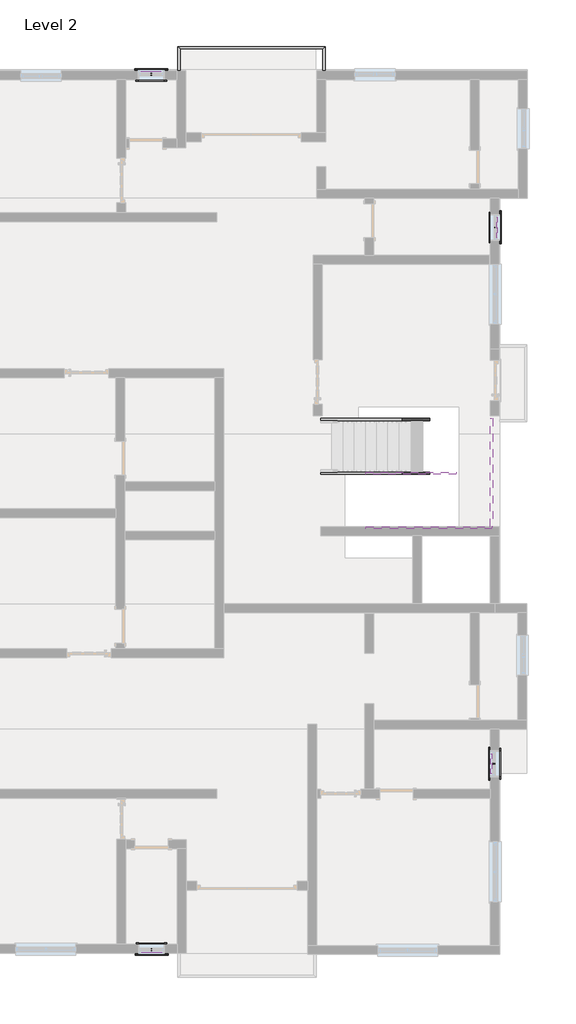
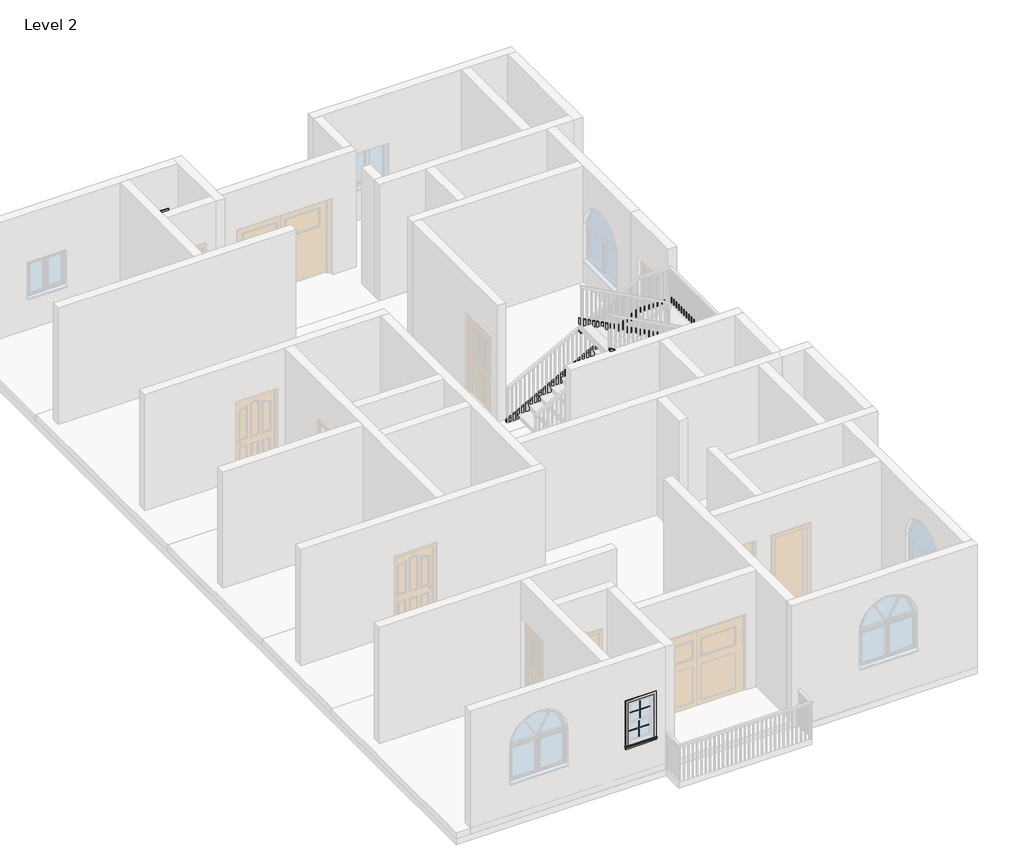
# One storey, part 7 of 7: 16 proxies, 5 members, 1 railing.
"""IFC4 building model written with IfcOpenShell, lengths in millimetres."""

from ifc_helpers import new_model, si_unit, frame, origin, place, context, project, spatial, polyline, outline, extrude, faceted_brep, transform, mapped, element, save
from components import muntin_pattern_2x2_muntin_pattern_2x2_eba6c5fb, trim_window_exterior_flat_with_sill_278e6a94, trim_window_interior_flat_picture_frame_e9fd5f45

model = new_model("IFC4")

# Units and contexts
model_context = context("Model", 3, world=origin())
ifc_project = project(units=[si_unit("LENGTHUNIT", "METRE", prefix="MILLI")], contexts=[model_context])

# Site, building, storey
site = spatial("IfcSite", under=ifc_project)
building = spatial("IfcBuilding", under=site)
storey = spatial("IfcBuildingStorey", under=building, Name="Level 2", Elevation=3048.0)

# Proxies
placement = place(None, origin())
muntin_pattern_2x2_muntin_pattern_2x2_shape = muntin_pattern_2x2_muntin_pattern_2x2_eba6c5fb(model_context)
element("IfcBuildingElementProxy", 1, Name="Muntin Pattern_2x2 : Muntin Pattern_2x2", ObjectType="Muntin Pattern_2x2 : Muntin Pattern_2x2", at=placement, inside=storey, context=model_context, shape_type="MappedRepresentation", body=[
    mapped(muntin_pattern_2x2_muntin_pattern_2x2_shape, transform((5828.2640963, 5846.2962251, 4518.025), x_axis=(0.0, -1.0, 0.0), y_axis=(1.0, 0.0, 0.0), z_axis=(0.0, 0.0, 1.0))),
])
element("IfcBuildingElementProxy", 2, Name="Muntin Pattern_2x2 : Muntin Pattern_2x2", ObjectType="Muntin Pattern_2x2 : Muntin Pattern_2x2", at=placement, inside=storey, context=model_context, shape_type="MappedRepresentation", body=[
    mapped(muntin_pattern_2x2_muntin_pattern_2x2_shape, transform((5783.8140963, 5846.2962251, 4038.6), x_axis=(0.0, -1.0, 0.0), y_axis=(1.0, 0.0, 0.0), z_axis=(0.0, 0.0, 1.0))),
])
element("IfcBuildingElementProxy", 3, Name="Muntin Pattern_2x2 : Muntin Pattern_2x2", ObjectType="Muntin Pattern_2x2 : Muntin Pattern_2x2", at=placement, inside=storey, context=model_context, shape_type="MappedRepresentation", body=[
    mapped(muntin_pattern_2x2_muntin_pattern_2x2_shape, transform((5694.9140963, -6313.9537749, 4518.025), x_axis=(0.0, 1.0, 0.0), y_axis=(-1.0, 0.0, 0.0), z_axis=(0.0, 0.0, 1.0))),
])
element("IfcBuildingElementProxy", 4, Name="Muntin Pattern_2x2 : Muntin Pattern_2x2", ObjectType="Muntin Pattern_2x2 : Muntin Pattern_2x2", at=placement, inside=storey, context=model_context, shape_type="MappedRepresentation", body=[
    mapped(muntin_pattern_2x2_muntin_pattern_2x2_shape, transform((5739.3640963, -6313.9537749, 4038.6), x_axis=(0.0, 1.0, 0.0), y_axis=(-1.0, 0.0, 0.0), z_axis=(0.0, 0.0, 1.0))),
])
element("IfcBuildingElementProxy", 5, Name="Muntin Pattern_2x2 : Muntin Pattern_2x2", ObjectType="Muntin Pattern_2x2 : Muntin Pattern_2x2", at=placement, inside=storey, context=model_context, shape_type="MappedRepresentation", body=[
    mapped(muntin_pattern_2x2_muntin_pattern_2x2_shape, transform((-2029.8609037, 9366.9277313, 4518.025), x_axis=(1.0, 0.0, 0.0), y_axis=(0.0, 1.0, 0.0), z_axis=(0.0, 0.0, 1.0))),
])
element("IfcBuildingElementProxy", 6, Name="Muntin Pattern_2x2 : Muntin Pattern_2x2", ObjectType="Muntin Pattern_2x2 : Muntin Pattern_2x2", at=placement, inside=storey, context=model_context, shape_type="MappedRepresentation", body=[
    mapped(muntin_pattern_2x2_muntin_pattern_2x2_shape, transform((-2029.8609037, 9322.4777313, 4038.6), x_axis=(1.0, 0.0, 0.0), y_axis=(0.0, 1.0, 0.0), z_axis=(0.0, 0.0, 1.0))),
])
element("IfcBuildingElementProxy", 7, Name="Muntin Pattern_2x2 : Muntin Pattern_2x2", ObjectType="Muntin Pattern_2x2 : Muntin Pattern_2x2", at=placement, inside=storey, context=model_context, shape_type="MappedRepresentation", body=[
    mapped(muntin_pattern_2x2_muntin_pattern_2x2_shape, transform((-2023.5109037, -10577.9787749, 4518.025), x_axis=(-1.0, 0.0, 0.0), y_axis=(0.0, -1.0, 0.0), z_axis=(0.0, 0.0, 1.0))),
])
element("IfcBuildingElementProxy", 8, Name="Muntin Pattern_2x2 : Muntin Pattern_2x2", ObjectType="Muntin Pattern_2x2 : Muntin Pattern_2x2", at=placement, inside=storey, context=model_context, shape_type="MappedRepresentation", body=[
    mapped(muntin_pattern_2x2_muntin_pattern_2x2_shape, transform((-2023.5109037, -10533.5287749, 4038.6), x_axis=(-1.0, 0.0, 0.0), y_axis=(0.0, -1.0, 0.0), z_axis=(0.0, 0.0, 1.0))),
])
trim_window_exterior_flat_with_sill_shape = trim_window_exterior_flat_with_sill_278e6a94(model_context)
element("IfcBuildingElementProxy", 9, Name="Trim-Window-Exterior-Flat : with Sill", ObjectType="Trim-Window-Exterior-Flat : with Sill", at=placement, inside=storey, context=model_context, shape_type="MappedRepresentation", body=[
    mapped(trim_window_exterior_flat_with_sill_shape, transform((5863.1890963, 5846.2962251, 5029.2), x_axis=(0.0, 1.0, 0.0), y_axis=(0.0, 0.0, 1.0), z_axis=(1.0, 0.0, 0.0))),
])
element("IfcBuildingElementProxy", 10, Name="Trim-Window-Exterior-Flat : with Sill", ObjectType="Trim-Window-Exterior-Flat : with Sill", at=placement, inside=storey, context=model_context, shape_type="MappedRepresentation", body=[
    mapped(trim_window_exterior_flat_with_sill_shape, transform((5659.9890963, -6313.9537749, 5029.2), x_axis=(0.0, -1.0, 0.0), y_axis=(0.0, 0.0, 1.0), z_axis=(-1.0, 0.0, 0.0))),
])
element("IfcBuildingElementProxy", 11, Name="Trim-Window-Exterior-Flat : with Sill", ObjectType="Trim-Window-Exterior-Flat : with Sill", at=placement, inside=storey, context=model_context, shape_type="MappedRepresentation", body=[
    mapped(trim_window_exterior_flat_with_sill_shape, transform((-2029.8609037, 9401.8527313, 5029.2), x_axis=(-1.0, 0.0, 0.0), y_axis=(0.0, 0.0, 1.0), z_axis=(0.0, 1.0, 0.0))),
])
element("IfcBuildingElementProxy", 12, Name="Trim-Window-Exterior-Flat : with Sill", ObjectType="Trim-Window-Exterior-Flat : with Sill", at=placement, inside=storey, context=model_context, shape_type="MappedRepresentation", body=[
    mapped(trim_window_exterior_flat_with_sill_shape, transform((-2023.5109037, -10612.9037749, 5029.2), x_axis=(1.0, 0.0, 0.0), y_axis=(0.0, 0.0, 1.0), z_axis=(0.0, -1.0, 0.0))),
])
trim_window_interior_flat_picture_frame_shape = trim_window_interior_flat_picture_frame_e9fd5f45(model_context)
element("IfcBuildingElementProxy", 13, Name="Trim-Window-Interior-Flat : Picture Frame", ObjectType="Trim-Window-Interior-Flat : Picture Frame", at=placement, inside=storey, context=model_context, shape_type="MappedRepresentation", body=[
    mapped(trim_window_interior_flat_picture_frame_shape, transform((5659.9890963, 5846.2962251, 5029.2), x_axis=(0.0, -1.0, 0.0), y_axis=(0.0, 0.0, 1.0), z_axis=(-1.0, 0.0, 0.0))),
])
element("IfcBuildingElementProxy", 14, Name="Trim-Window-Interior-Flat : Picture Frame", ObjectType="Trim-Window-Interior-Flat : Picture Frame", at=placement, inside=storey, context=model_context, shape_type="MappedRepresentation", body=[
    mapped(trim_window_interior_flat_picture_frame_shape, transform((5863.1890963, -6313.9537749, 5029.2), x_axis=(0.0, 1.0, 0.0), y_axis=(0.0, 0.0, 1.0), z_axis=(1.0, 0.0, 0.0))),
])
element("IfcBuildingElementProxy", 15, Name="Trim-Window-Interior-Flat : Picture Frame", ObjectType="Trim-Window-Interior-Flat : Picture Frame", at=placement, inside=storey, context=model_context, shape_type="MappedRepresentation", body=[
    mapped(trim_window_interior_flat_picture_frame_shape, transform((-2029.8609037, 9198.6527313, 5029.2), x_axis=(1.0, 0.0, 0.0), y_axis=(0.0, 0.0, 1.0), z_axis=(0.0, -1.0, 0.0))),
])
element("IfcBuildingElementProxy", 16, Name="Trim-Window-Interior-Flat : Picture Frame", ObjectType="Trim-Window-Interior-Flat : Picture Frame", at=placement, inside=storey, context=model_context, shape_type="MappedRepresentation", body=[
    mapped(trim_window_interior_flat_picture_frame_shape, transform((-2023.5109037, -10409.7037749, 5029.2), x_axis=(-1.0, 0.0, 0.0), y_axis=(0.0, 0.0, 1.0), z_axis=(0.0, 1.0, 0.0))),
])

# Members
element("IfcMember", 17, ObjectType="Stringer - 2\" Width", at=placement, inside=storey, context=model_context, shape_type="SweptSolid", body=[
    extrude(outline(polyline([(3255.4423129, 1811.8890963), (3048.0, 1811.8890963), (3048.0, 2068.9379367), (4925.2909091, 5536.6829612), (4925.2909091, 4896.4452154), (3255.4423129, 1811.8890963)])), frame((0.0, 1464.7962251, 0.0), z_axis=(0.0, 1.0, 0.0), x_axis=(0.0, 0.0, 1.0)), (0.0, 0.0, 1.0), 50.8),
])
element("IfcMember", 18, ObjectType="Stringer - 2\" Width", at=placement, inside=storey, context=model_context, shape_type="SweptSolid", body=[
    extrude(outline(polyline([(5659.9890963, 1515.5962251), (5710.7890963, 1515.5962251), (5710.7890963, -935.5037749), (5659.9890963, -935.5037749), (5659.9890963, 1515.5962251)])), frame((0.0, 0.0, 4620.4909091), z_axis=(0.0, 0.0, 1.0), x_axis=(1.0, 0.0, 0.0)), (0.0, 0.0, 1.0), 304.8),
])
element("IfcMember", 19, ObjectType="Stringer - 2\" Width", at=placement, inside=storey, context=model_context, shape_type="SweptSolid", body=[
    extrude(outline(polyline([(4620.4909091, 5687.6636359), (6162.0362324, 2827.8890963), (5815.7736638, 2827.8890963), (4620.4909091, 5045.2998579), (4620.4909091, 5687.6636359)])), frame((0.0, -986.3037749, 0.0), z_axis=(0.0, 1.0, 0.0), x_axis=(0.0, 0.0, 1.0)), (0.0, 0.0, 1.0), 50.8),
])
element("IfcMember", 20, ObjectType="Stringer - 2\" Width", at=placement, inside=storey, context=model_context, shape_type="SweptSolid", body=[
    extrude(outline(polyline([(3255.4423129, 1811.8890963), (3048.0, 1811.8890963), (3048.0, 2068.9379367), (4542.8485088, 4830.2326586), (4889.4462232, 4830.2326586), (3255.4423129, 1811.8890963)])), frame((0.0, 245.5962251, 0.0), z_axis=(0.0, 1.0, 0.0), x_axis=(0.0, 0.0, 1.0)), (0.0, 0.0, 1.0), 50.8),
])
element("IfcMember", 21, ObjectType="Stringer - 2\" Width", at=placement, inside=storey, context=model_context, shape_type="SweptSolid", body=[
    extrude(outline(polyline([(4709.0382157, 4881.0326586), (5055.3007843, 4881.0326586), (6162.0362324, 2827.8890963), (5815.7736638, 2827.8890963), (4709.0382157, 4881.0326586)])), frame((0.0, 245.5962251, 0.0), z_axis=(0.0, 1.0, 0.0), x_axis=(0.0, 0.0, 1.0)), (0.0, 0.0, 1.0), 50.8),
])

# Railing
element("IfcRailing", 22, ObjectType="Handrail - Rectangular", at=placement, inside=storey, context=model_context, shape_type="SolidModel", body=[
    faceted_brep([(-1426.6109037, 9402.2962251, 3962.4), (-1426.6109037, 9402.2962251, 3911.6), (-1375.8109037, 9402.2962251, 3911.6), (-1375.8109037, 9402.2962251, 3962.4), (-1426.6109037, 9948.3962251, 3962.4), (-1426.6109037, 9948.3962251, 3911.6), (-1375.8109037, 9897.5962251, 3911.6), (-1375.8109037, 9897.5962251, 3962.4), (1913.4890963, 9948.3962251, 3962.4), (1913.4890963, 9948.3962251, 3911.6), (1862.6890963, 9897.5962251, 3911.6), (1862.6890963, 9897.5962251, 3962.4), (1913.4890963, 9402.2962251, 3962.4), (1862.6890963, 9402.2962251, 3962.4), (1862.6890963, 9402.2962251, 3911.6), (1913.4890963, 9402.2962251, 3911.6)], [[[0, 1, 2, 3]], [[1, 0, 4, 5]], [[2, 1, 5, 6]], [[3, 2, 6, 7]], [[0, 3, 7, 4]], [[5, 4, 8, 9]], [[6, 5, 9, 10]], [[7, 6, 10, 11]], [[4, 7, 11, 8]], [[12, 13, 14, 15]], [[9, 8, 12, 15]], [[10, 9, 15, 14]], [[11, 10, 14, 13]], [[8, 11, 13, 12]]]),
    extrude(outline(polyline([(1878.5640963, 9424.5212251), (1897.6140963, 9424.5212251), (1897.6140963, 9405.4712251), (1878.5640963, 9405.4712251), (1878.5640963, 9424.5212251)])), frame((0.0, 0.0, 3048.0), z_axis=(0.0, 0.0, 1.0), x_axis=(1.0, 0.0, 0.0)), (0.0, 0.0, 1.0), 863.6),
    extrude(outline(polyline([(1878.5640963, 9526.1212251), (1897.6140963, 9526.1212251), (1897.6140963, 9507.0712251), (1878.5640963, 9507.0712251), (1878.5640963, 9526.1212251)])), frame((0.0, 0.0, 3048.0), z_axis=(0.0, 0.0, 1.0), x_axis=(1.0, 0.0, 0.0)), (0.0, 0.0, 1.0), 863.6),
    extrude(outline(polyline([(1878.5640963, 9627.7212251), (1897.6140963, 9627.7212251), (1897.6140963, 9608.6712251), (1878.5640963, 9608.6712251), (1878.5640963, 9627.7212251)])), frame((0.0, 0.0, 3048.0), z_axis=(0.0, 0.0, 1.0), x_axis=(1.0, 0.0, 0.0)), (0.0, 0.0, 1.0), 863.6),
    extrude(outline(polyline([(1878.5640963, 9729.3212251), (1897.6140963, 9729.3212251), (1897.6140963, 9710.2712251), (1878.5640963, 9710.2712251), (1878.5640963, 9729.3212251)])), frame((0.0, 0.0, 3048.0), z_axis=(0.0, 0.0, 1.0), x_axis=(1.0, 0.0, 0.0)), (0.0, 0.0, 1.0), 863.6),
    extrude(outline(polyline([(1878.5640963, 9830.9212251), (1897.6140963, 9830.9212251), (1897.6140963, 9811.8712251), (1878.5640963, 9811.8712251), (1878.5640963, 9830.9212251)])), frame((0.0, 0.0, 3048.0), z_axis=(0.0, 0.0, 1.0), x_axis=(1.0, 0.0, 0.0)), (0.0, 0.0, 1.0), 863.6),
    extrude(outline(polyline([(1840.4640963, 9913.4712251), (1840.4640963, 9932.5212251), (1859.5140963, 9932.5212251), (1859.5140963, 9913.4712251), (1840.4640963, 9913.4712251)])), frame((0.0, 0.0, 3048.0), z_axis=(0.0, 0.0, 1.0), x_axis=(1.0, 0.0, 0.0)), (0.0, 0.0, 1.0), 863.6),
    extrude(outline(polyline([(1738.8640963, 9913.4712251), (1738.8640963, 9932.5212251), (1757.9140963, 9932.5212251), (1757.9140963, 9913.4712251), (1738.8640963, 9913.4712251)])), frame((0.0, 0.0, 3048.0), z_axis=(0.0, 0.0, 1.0), x_axis=(1.0, 0.0, 0.0)), (0.0, 0.0, 1.0), 863.6),
    extrude(outline(polyline([(1637.2640963, 9913.4712251), (1637.2640963, 9932.5212251), (1656.3140963, 9932.5212251), (1656.3140963, 9913.4712251), (1637.2640963, 9913.4712251)])), frame((0.0, 0.0, 3048.0), z_axis=(0.0, 0.0, 1.0), x_axis=(1.0, 0.0, 0.0)), (0.0, 0.0, 1.0), 863.6),
    extrude(outline(polyline([(1535.6640963, 9913.4712251), (1535.6640963, 9932.5212251), (1554.7140963, 9932.5212251), (1554.7140963, 9913.4712251), (1535.6640963, 9913.4712251)])), frame((0.0, 0.0, 3048.0), z_axis=(0.0, 0.0, 1.0), x_axis=(1.0, 0.0, 0.0)), (0.0, 0.0, 1.0), 863.6),
    extrude(outline(polyline([(1434.0640963, 9913.4712251), (1434.0640963, 9932.5212251), (1453.1140963, 9932.5212251), (1453.1140963, 9913.4712251), (1434.0640963, 9913.4712251)])), frame((0.0, 0.0, 3048.0), z_axis=(0.0, 0.0, 1.0), x_axis=(1.0, 0.0, 0.0)), (0.0, 0.0, 1.0), 863.6),
    extrude(outline(polyline([(1332.4640963, 9913.4712251), (1332.4640963, 9932.5212251), (1351.5140963, 9932.5212251), (1351.5140963, 9913.4712251), (1332.4640963, 9913.4712251)])), frame((0.0, 0.0, 3048.0), z_axis=(0.0, 0.0, 1.0), x_axis=(1.0, 0.0, 0.0)), (0.0, 0.0, 1.0), 863.6),
    extrude(outline(polyline([(1230.8640963, 9913.4712251), (1230.8640963, 9932.5212251), (1249.9140963, 9932.5212251), (1249.9140963, 9913.4712251), (1230.8640963, 9913.4712251)])), frame((0.0, 0.0, 3048.0), z_axis=(0.0, 0.0, 1.0), x_axis=(1.0, 0.0, 0.0)), (0.0, 0.0, 1.0), 863.6),
    extrude(outline(polyline([(1129.2640963, 9913.4712251), (1129.2640963, 9932.5212251), (1148.3140963, 9932.5212251), (1148.3140963, 9913.4712251), (1129.2640963, 9913.4712251)])), frame((0.0, 0.0, 3048.0), z_axis=(0.0, 0.0, 1.0), x_axis=(1.0, 0.0, 0.0)), (0.0, 0.0, 1.0), 863.6),
    extrude(outline(polyline([(1027.6640963, 9913.4712251), (1027.6640963, 9932.5212251), (1046.7140963, 9932.5212251), (1046.7140963, 9913.4712251), (1027.6640963, 9913.4712251)])), frame((0.0, 0.0, 3048.0), z_axis=(0.0, 0.0, 1.0), x_axis=(1.0, 0.0, 0.0)), (0.0, 0.0, 1.0), 863.6),
    extrude(outline(polyline([(926.0640963, 9913.4712251), (926.0640963, 9932.5212251), (945.1140963, 9932.5212251), (945.1140963, 9913.4712251), (926.0640963, 9913.4712251)])), frame((0.0, 0.0, 3048.0), z_axis=(0.0, 0.0, 1.0), x_axis=(1.0, 0.0, 0.0)), (0.0, 0.0, 1.0), 863.6),
    extrude(outline(polyline([(824.4640963, 9913.4712251), (824.4640963, 9932.5212251), (843.5140963, 9932.5212251), (843.5140963, 9913.4712251), (824.4640963, 9913.4712251)])), frame((0.0, 0.0, 3048.0), z_axis=(0.0, 0.0, 1.0), x_axis=(1.0, 0.0, 0.0)), (0.0, 0.0, 1.0), 863.6),
    extrude(outline(polyline([(722.8640963, 9913.4712251), (722.8640963, 9932.5212251), (741.9140963, 9932.5212251), (741.9140963, 9913.4712251), (722.8640963, 9913.4712251)])), frame((0.0, 0.0, 3048.0), z_axis=(0.0, 0.0, 1.0), x_axis=(1.0, 0.0, 0.0)), (0.0, 0.0, 1.0), 863.6),
    extrude(outline(polyline([(621.2640963, 9913.4712251), (621.2640963, 9932.5212251), (640.3140963, 9932.5212251), (640.3140963, 9913.4712251), (621.2640963, 9913.4712251)])), frame((0.0, 0.0, 3048.0), z_axis=(0.0, 0.0, 1.0), x_axis=(1.0, 0.0, 0.0)), (0.0, 0.0, 1.0), 863.6),
    extrude(outline(polyline([(519.6640963, 9913.4712251), (519.6640963, 9932.5212251), (538.7140963, 9932.5212251), (538.7140963, 9913.4712251), (519.6640963, 9913.4712251)])), frame((0.0, 0.0, 3048.0), z_axis=(0.0, 0.0, 1.0), x_axis=(1.0, 0.0, 0.0)), (0.0, 0.0, 1.0), 863.6),
    extrude(outline(polyline([(418.0640963, 9913.4712251), (418.0640963, 9932.5212251), (437.1140963, 9932.5212251), (437.1140963, 9913.4712251), (418.0640963, 9913.4712251)])), frame((0.0, 0.0, 3048.0), z_axis=(0.0, 0.0, 1.0), x_axis=(1.0, 0.0, 0.0)), (0.0, 0.0, 1.0), 863.6),
    extrude(outline(polyline([(316.4640963, 9913.4712251), (316.4640963, 9932.5212251), (335.5140963, 9932.5212251), (335.5140963, 9913.4712251), (316.4640963, 9913.4712251)])), frame((0.0, 0.0, 3048.0), z_axis=(0.0, 0.0, 1.0), x_axis=(1.0, 0.0, 0.0)), (0.0, 0.0, 1.0), 863.6),
    extrude(outline(polyline([(214.8640963, 9913.4712251), (214.8640963, 9932.5212251), (233.9140963, 9932.5212251), (233.9140963, 9913.4712251), (214.8640963, 9913.4712251)])), frame((0.0, 0.0, 3048.0), z_axis=(0.0, 0.0, 1.0), x_axis=(1.0, 0.0, 0.0)), (0.0, 0.0, 1.0), 863.6),
    extrude(outline(polyline([(113.2640963, 9913.4712251), (113.2640963, 9932.5212251), (132.3140963, 9932.5212251), (132.3140963, 9913.4712251), (113.2640963, 9913.4712251)])), frame((0.0, 0.0, 3048.0), z_axis=(0.0, 0.0, 1.0), x_axis=(1.0, 0.0, 0.0)), (0.0, 0.0, 1.0), 863.6),
    extrude(outline(polyline([(11.6640963, 9913.4712251), (11.6640963, 9932.5212251), (30.7140963, 9932.5212251), (30.7140963, 9913.4712251), (11.6640963, 9913.4712251)])), frame((0.0, 0.0, 3048.0), z_axis=(0.0, 0.0, 1.0), x_axis=(1.0, 0.0, 0.0)), (0.0, 0.0, 1.0), 863.6),
    extrude(outline(polyline([(-89.9359037, 9913.4712251), (-89.9359037, 9932.5212251), (-70.8859037, 9932.5212251), (-70.8859037, 9913.4712251), (-89.9359037, 9913.4712251)])), frame((0.0, 0.0, 3048.0), z_axis=(0.0, 0.0, 1.0), x_axis=(1.0, 0.0, 0.0)), (0.0, 0.0, 1.0), 863.6),
    extrude(outline(polyline([(-191.5359037, 9913.4712251), (-191.5359037, 9932.5212251), (-172.4859037, 9932.5212251), (-172.4859037, 9913.4712251), (-191.5359037, 9913.4712251)])), frame((0.0, 0.0, 3048.0), z_axis=(0.0, 0.0, 1.0), x_axis=(1.0, 0.0, 0.0)), (0.0, 0.0, 1.0), 863.6),
    extrude(outline(polyline([(-293.1359037, 9913.4712251), (-293.1359037, 9932.5212251), (-274.0859037, 9932.5212251), (-274.0859037, 9913.4712251), (-293.1359037, 9913.4712251)])), frame((0.0, 0.0, 3048.0), z_axis=(0.0, 0.0, 1.0), x_axis=(1.0, 0.0, 0.0)), (0.0, 0.0, 1.0), 863.6),
    extrude(outline(polyline([(-394.7359037, 9913.4712251), (-394.7359037, 9932.5212251), (-375.6859037, 9932.5212251), (-375.6859037, 9913.4712251), (-394.7359037, 9913.4712251)])), frame((0.0, 0.0, 3048.0), z_axis=(0.0, 0.0, 1.0), x_axis=(1.0, 0.0, 0.0)), (0.0, 0.0, 1.0), 863.6),
    extrude(outline(polyline([(-496.3359037, 9913.4712251), (-496.3359037, 9932.5212251), (-477.2859037, 9932.5212251), (-477.2859037, 9913.4712251), (-496.3359037, 9913.4712251)])), frame((0.0, 0.0, 3048.0), z_axis=(0.0, 0.0, 1.0), x_axis=(1.0, 0.0, 0.0)), (0.0, 0.0, 1.0), 863.6),
    extrude(outline(polyline([(-597.9359037, 9913.4712251), (-597.9359037, 9932.5212251), (-578.8859037, 9932.5212251), (-578.8859037, 9913.4712251), (-597.9359037, 9913.4712251)])), frame((0.0, 0.0, 3048.0), z_axis=(0.0, 0.0, 1.0), x_axis=(1.0, 0.0, 0.0)), (0.0, 0.0, 1.0), 863.6),
    extrude(outline(polyline([(-699.5359037, 9913.4712251), (-699.5359037, 9932.5212251), (-680.4859037, 9932.5212251), (-680.4859037, 9913.4712251), (-699.5359037, 9913.4712251)])), frame((0.0, 0.0, 3048.0), z_axis=(0.0, 0.0, 1.0), x_axis=(1.0, 0.0, 0.0)), (0.0, 0.0, 1.0), 863.6),
    extrude(outline(polyline([(-801.1359037, 9913.4712251), (-801.1359037, 9932.5212251), (-782.0859037, 9932.5212251), (-782.0859037, 9913.4712251), (-801.1359037, 9913.4712251)])), frame((0.0, 0.0, 3048.0), z_axis=(0.0, 0.0, 1.0), x_axis=(1.0, 0.0, 0.0)), (0.0, 0.0, 1.0), 863.6),
    extrude(outline(polyline([(-902.7359037, 9913.4712251), (-902.7359037, 9932.5212251), (-883.6859037, 9932.5212251), (-883.6859037, 9913.4712251), (-902.7359037, 9913.4712251)])), frame((0.0, 0.0, 3048.0), z_axis=(0.0, 0.0, 1.0), x_axis=(1.0, 0.0, 0.0)), (0.0, 0.0, 1.0), 863.6),
    extrude(outline(polyline([(-1004.3359037, 9913.4712251), (-1004.3359037, 9932.5212251), (-985.2859037, 9932.5212251), (-985.2859037, 9913.4712251), (-1004.3359037, 9913.4712251)])), frame((0.0, 0.0, 3048.0), z_axis=(0.0, 0.0, 1.0), x_axis=(1.0, 0.0, 0.0)), (0.0, 0.0, 1.0), 863.6),
    extrude(outline(polyline([(-1105.9359037, 9913.4712251), (-1105.9359037, 9932.5212251), (-1086.8859037, 9932.5212251), (-1086.8859037, 9913.4712251), (-1105.9359037, 9913.4712251)])), frame((0.0, 0.0, 3048.0), z_axis=(0.0, 0.0, 1.0), x_axis=(1.0, 0.0, 0.0)), (0.0, 0.0, 1.0), 863.6),
    extrude(outline(polyline([(-1207.5359037, 9913.4712251), (-1207.5359037, 9932.5212251), (-1188.4859037, 9932.5212251), (-1188.4859037, 9913.4712251), (-1207.5359037, 9913.4712251)])), frame((0.0, 0.0, 3048.0), z_axis=(0.0, 0.0, 1.0), x_axis=(1.0, 0.0, 0.0)), (0.0, 0.0, 1.0), 863.6),
    extrude(outline(polyline([(-1309.1359037, 9913.4712251), (-1309.1359037, 9932.5212251), (-1290.0859037, 9932.5212251), (-1290.0859037, 9913.4712251), (-1309.1359037, 9913.4712251)])), frame((0.0, 0.0, 3048.0), z_axis=(0.0, 0.0, 1.0), x_axis=(1.0, 0.0, 0.0)), (0.0, 0.0, 1.0), 863.6),
    extrude(outline(polyline([(-1391.6859037, 9900.7712251), (-1410.7359037, 9900.7712251), (-1410.7359037, 9919.8212251), (-1391.6859037, 9919.8212251), (-1391.6859037, 9900.7712251)])), frame((0.0, 0.0, 3048.0), z_axis=(0.0, 0.0, 1.0), x_axis=(1.0, 0.0, 0.0)), (0.0, 0.0, 1.0), 863.6),
    extrude(outline(polyline([(-1391.6859037, 9799.1712251), (-1410.7359037, 9799.1712251), (-1410.7359037, 9818.2212251), (-1391.6859037, 9818.2212251), (-1391.6859037, 9799.1712251)])), frame((0.0, 0.0, 3048.0), z_axis=(0.0, 0.0, 1.0), x_axis=(1.0, 0.0, 0.0)), (0.0, 0.0, 1.0), 863.6),
    extrude(outline(polyline([(-1391.6859037, 9697.5712251), (-1410.7359037, 9697.5712251), (-1410.7359037, 9716.6212251), (-1391.6859037, 9716.6212251), (-1391.6859037, 9697.5712251)])), frame((0.0, 0.0, 3048.0), z_axis=(0.0, 0.0, 1.0), x_axis=(1.0, 0.0, 0.0)), (0.0, 0.0, 1.0), 863.6),
    extrude(outline(polyline([(-1391.6859037, 9595.9712251), (-1410.7359037, 9595.9712251), (-1410.7359037, 9615.0212251), (-1391.6859037, 9615.0212251), (-1391.6859037, 9595.9712251)])), frame((0.0, 0.0, 3048.0), z_axis=(0.0, 0.0, 1.0), x_axis=(1.0, 0.0, 0.0)), (0.0, 0.0, 1.0), 863.6),
    extrude(outline(polyline([(-1391.6859037, 9494.3712251), (-1410.7359037, 9494.3712251), (-1410.7359037, 9513.4212251), (-1391.6859037, 9513.4212251), (-1391.6859037, 9494.3712251)])), frame((0.0, 0.0, 3048.0), z_axis=(0.0, 0.0, 1.0), x_axis=(1.0, 0.0, 0.0)), (0.0, 0.0, 1.0), 863.6),
    extrude(outline(polyline([(1878.5640963, 9913.4712251), (1878.5640963, 9932.5212251), (1897.6140963, 9932.5212251), (1897.6140963, 9913.4712251), (1878.5640963, 9913.4712251)])), frame((0.0, 0.0, 3048.0), z_axis=(0.0, 0.0, 1.0), x_axis=(1.0, 0.0, 0.0)), (0.0, 0.0, 1.0), 863.6),
    extrude(outline(polyline([(-1391.6859037, 9913.4712251), (-1410.7359037, 9913.4712251), (-1410.7359037, 9932.5212251), (-1391.6859037, 9932.5212251), (-1391.6859037, 9913.4712251)])), frame((0.0, 0.0, 3048.0), z_axis=(0.0, 0.0, 1.0), x_axis=(1.0, 0.0, 0.0)), (0.0, 0.0, 1.0), 863.6),
    extrude(outline(polyline([(1878.5640963, 9421.3462251), (1897.6140963, 9421.3462251), (1897.6140963, 9402.2962251), (1878.5640963, 9402.2962251), (1878.5640963, 9421.3462251)])), frame((0.0, 0.0, 3048.0), z_axis=(0.0, 0.0, 1.0), x_axis=(1.0, 0.0, 0.0)), (0.0, 0.0, 1.0), 863.6),
    extrude(outline(polyline([(-1391.6859037, 9402.2962251), (-1410.7359037, 9402.2962251), (-1410.7359037, 9421.3462251), (-1391.6859037, 9421.3462251), (-1391.6859037, 9402.2962251)])), frame((0.0, 0.0, 3048.0), z_axis=(0.0, 0.0, 1.0), x_axis=(1.0, 0.0, 0.0)), (0.0, 0.0, 1.0), 863.6),
])

save(model, "model.ifc")

# Revit data of these elements
# Type "Muntin Pattern_2x2 : Muntin Pattern_2x2"
#   Width [instance default] = 4' - 0"
#   Thickness = 0' - 0 1/2"
#   Height [instance default] = 4' - 0"
#   Distance = 0' - 0 3/4"
#   Interior Material [instance default] = none
#   Exterior Material [instance default] = none
#   Default Elevation = 0
# Type "Trim-Window-Exterior-Flat : with Sill"
#   Trim Width = 0' - 2 1/4"
#   Trim Thickness_Picture Frame = 0' - 1 1/4"
#   Trim Thickness_with Sill = 0' - 0 3/4"
#   Sill Thickness = 0' - 1 1/4"
#   Opening Width [instance default] = 2' - 0"
#   Opening Height [instance default] = 3' - 0"
#   Default Elevation = 4' - 0"
#   Sill = yes
#   Picture Frame = no
#   Trim Material [instance default] = none
# Type "Trim-Window-Interior-Flat : Picture Frame"
#   Trim Thickness_Picture Frame = 0' - 1 1/4"
#   Trim Width = 0' - 2 1/4"
#   Trim Thickness_with Sill = 0' - 0 3/4"
#   Sill Thickness = 0' - 1 1/4"
#   Opening Width [instance default] = 2' - 0"
#   Opening Height [instance default] = 3' - 0"
#   Default Elevation = 4' - 0"
#   Sill = no
#   Picture Frame = yes
#   Trim Material [instance default] = none
# Type "Handrail - Rectangular"
#   Assembly Code = "C2010400"
#   built-in parameter 1008612 = 0.0416667 (stored number, unit not read)
#   built-in parameter 1008611 = 0.0416667 (stored number, unit not read)
#   built-in parameter 1008609 = 0.333333 (stored number, unit not read)
#   built-in parameter 1008604 = 0.166667 (stored number, unit not read)
#   built-in parameter 1008603 = 0.166667 (stored number, unit not read)
#   Railing Height = 3' - 0"
#   built-in parameter 1008630 = 2
#   built-in parameter 1008610 = 2
#   built-in parameter 1008618 = Baluster - Square : 3/4"
# Elements 1, 2, 3, 4, 5, 6, 7, 8 (IfcBuildingElementProxy, "Muntin Pattern_2x2 : Muntin Pattern_2x2")
#   Width = 1' - 6"
#   Height = 1' - 5 1/8"
#   Interior Material = Wood - Stained
#   Exterior Material = Clad - White
#   Phase Created = New Construction
#   Materials on its faces: "Clad - White", "Wood - Stained"
# Elements 9, 10, 11, 12 (IfcBuildingElementProxy, "Trim-Window-Exterior-Flat : with Sill")
#   Opening Width = 2' - 0"
#   Opening Height = 3' - 6"
#   Trim Material = Clad - White
#   Phase Created = New Construction
#   Materials on its faces: "Clad - White"
# Elements 13, 14, 15, 16 (IfcBuildingElementProxy, "Trim-Window-Interior-Flat : Picture Frame")
#   Opening Width = 2' - 0"
#   Opening Height = 3' - 6"
#   Trim Material = Wood - Stained
#   Phase Created = New Construction
#   Materials on its faces: "Wood - Stained"
# Elements 17, 18, 19, 20, 21 (IfcMember, "Stringer - 2\" Width")
#   Phase Created = New Construction
# Element 22 (IfcRailing, "Handrail - Rectangular")
#   Phase Created = New Construction
# Materials
#   "Clad - White": class "Wood", colour RGB 242 242 238, transparency 0, Cost = 0
#   "Wood - Stained": class "Wood", colour RGB 224 178 126, transparency 0, Cost = 0
